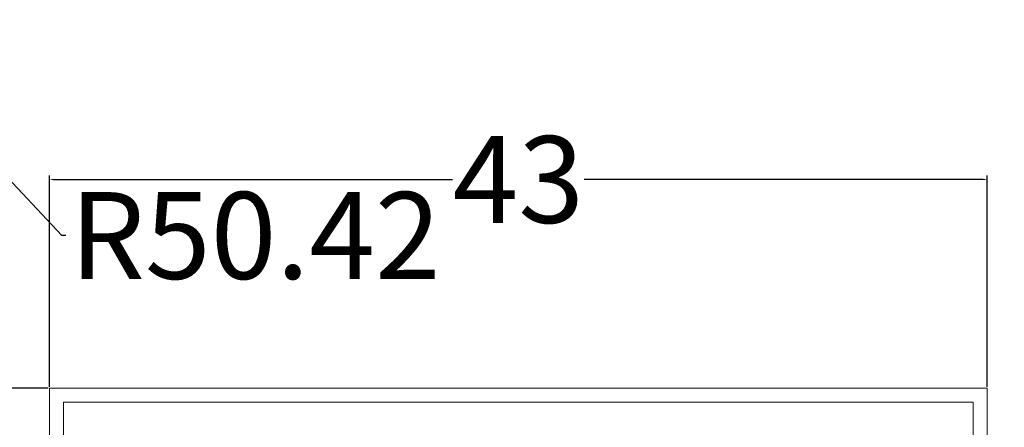
# Model space of a CAD drawing. Units: inches. Extents: x 1291 to 2095, y 532 to 1090.
# Tile 8 of 14: x 1618 to 1663, y 798 to 817. Entities that reach past the tile are written whole.
import ezdxf

# ---------------------------------------------------------------- set-up
doc = ezdxf.new("R2010")
doc.units = ezdxf.units.IN
doc.header["$MEASUREMENT"] = 0
doc.layers.add('A-ANNO-DIMS', color=2, linetype='Continuous', lineweight=18)
doc.layers.add('A-FURN', color=8, linetype='Continuous', lineweight=18)
doc.styles.get("Standard").update_dxf_attribs({"font": 'arial.ttf'})
doc.dimstyles.get("Standard").update_dxf_attribs({"dimtxt": 4, "dimasz": 0.18, "dimexe": 0.18, "dimexo": 0.0625, "dimgap": 0.09, "dimtad": 0, "dimtih": 1, "dimtoh": 1, "dimdec": 0, "dimrnd": 6, "dimzin": 0, "dimdsep": 46, "dimlunit": 3, "dimtxsty": 'Standard', "dimcen": 0.09, "dimadec": 0, "dimazin": 0, "dimtfac": 1, "dimtdec": 0, "dimtofl": 0, "dimtmove": 0, "dimatfit": 3, "dimfxl": 1, "dimtolj": 1, "dimtzin": 0, "dimarcsym": 0})

# ---------------------------------------------------------------- blocks, each defined once
blk = doc.blocks.new('A$C73B76B3A')
for p, q in [((0, 0), (0, 2)), ((1.35, 0), (1.35, 2)), ((0.02, 0.02), (0.02, 1.98)), ((1.33, 1.98), (1.33, 0.02)), ((1.33, 0.02), (0.02, 0.02)), ((1.35, 0), (0, 0))]:
    blk.add_line(p, q)
blk = doc.blocks.new('*D30')
at = {"layer": 'A-ANNO-DIMS', "color": 0, "lineweight": -2, "transparency": 16777216}
for p, q in [((1618.87, 799.814), (1609.145, 799.814)), ((1609.325, 799.634), (1609.325, 769.922)), ((1609.325, 735.946), (1609.325, 765.658)), ((1618.87, 735.766), (1609.145, 735.766))]:
    blk.add_line(p, q, dxfattribs=at)
at = {"layer": 'A-ANNO-DIMS', "color": 0, "transparency": 16777216}
for points in [[(1609.295, 799.634), (1609.355, 799.634), (1609.325, 799.814)], [(1609.295, 735.946), (1609.355, 735.946), (1609.325, 735.766)]]:
    blk.add_solid(points, dxfattribs=at)
at = {"layer": 'Defpoints', "color": 0, "transparency": 16777216}
for p in [(1618.932, 799.814), (1609.325, 735.766), (1618.932, 735.766)]:
    blk.add_point(p, dxfattribs=at)
at = {"layer": 'A-ANNO-DIMS', "color": 0, "transparency": 16777216, "insert": (1609.325, 767.79), "char_height": 4, "attachment_point": 5}
blk.add_mtext('\\A1;BED 64', dxfattribs=at)
blk = doc.blocks.new('*D31')
at = {"layer": 'A-ANNO-DIMS', "color": 0, "lineweight": -2, "transparency": 16777216}
for p, q in [((1618.932, 799.877), (1618.932, 809.602)), ((1619.112, 809.422), (1637.513, 809.422)), ((1661.985, 809.422), (1643.584, 809.422)), ((1662.165, 799.877), (1662.165, 809.602))]:
    blk.add_line(p, q, dxfattribs=at)
at = {"layer": 'A-ANNO-DIMS', "color": 0, "transparency": 16777216}
for points in [[(1619.112, 809.452), (1619.112, 809.392), (1618.932, 809.422)], [(1661.985, 809.452), (1661.985, 809.392), (1662.165, 809.422)]]:
    blk.add_solid(points, dxfattribs=at)
at = {"layer": 'Defpoints', "color": 0, "transparency": 16777216}
for p in [(1618.932, 809.422), (1618.932, 799.814), (1662.165, 799.814)]:
    blk.add_point(p, dxfattribs=at)
at = {"layer": 'A-ANNO-DIMS', "color": 0, "transparency": 16777216, "insert": (1640.548, 809.422), "char_height": 4, "attachment_point": 5}
blk.add_mtext('\\A1;43', dxfattribs=at)
blk = doc.blocks.new('*D46')
at = {"layer": 'A-ANNO-DIMS', "color": 0, "lineweight": -2, "transparency": 16777216}
for p, q in [((1600.27, 579.843), (1600.27, 1087.16)), ((1600.45, 1086.98), (1636.471, 1086.98)), ((1685.404, 1086.98), (1649.383, 1086.98)), ((1685.584, 579.843), (1685.584, 1087.16))]:
    blk.add_line(p, q, dxfattribs=at)
at = {"layer": 'A-ANNO-DIMS', "color": 0, "transparency": 16777216}
for points in [[(1600.45, 1087.01), (1600.45, 1086.95), (1600.27, 1086.98)], [(1685.404, 1087.01), (1685.404, 1086.95), (1685.584, 1086.98)]]:
    blk.add_solid(points, dxfattribs=at)
at = {"layer": 'Defpoints', "color": 0, "transparency": 16777216}
for p in [(1685.584, 1086.98), (1600.27, 579.78), (1685.584, 579.78)]:
    blk.add_point(p, dxfattribs=at)
at = {"layer": 'A-ANNO-DIMS', "color": 0, "transparency": 16777216, "insert": (1642.927, 1086.98), "char_height": 4, "attachment_point": 5}
blk.add_mtext('\\A1;85.31', dxfattribs=at)
blk = doc.blocks.new('*D49')
at = {"layer": 'A-ANNO-DIMS', "color": 0, "lineweight": -2, "transparency": 16777216}
for p, q in [((1694.074, 852.718), (1694.074, 534.4)), ((1586.074, 816.718), (1586.074, 534.4)), ((1586.254, 534.58), (1635.749, 534.58)), ((1693.894, 534.58), (1644.398, 534.58))]:
    blk.add_line(p, q, dxfattribs=at)
at = {"layer": 'A-ANNO-DIMS', "color": 0, "transparency": 16777216}
for points in [[(1586.254, 534.61), (1586.254, 534.55), (1586.074, 534.58)], [(1693.894, 534.61), (1693.894, 534.55), (1694.074, 534.58)]]:
    blk.add_solid(points, dxfattribs=at)
at = {"layer": 'Defpoints', "color": 0, "transparency": 16777216}
for p in [(1694.074, 852.78), (1586.074, 816.78), (1694.074, 534.58)]:
    blk.add_point(p, dxfattribs=at)
at = {"layer": 'A-ANNO-DIMS', "color": 0, "transparency": 16777216, "insert": (1640.074, 534.58), "char_height": 4, "attachment_point": 5}
blk.add_mtext('\\A1;108', dxfattribs=at)
blk = doc.blocks.new('*D51')
at = {"layer": 'A-ANNO-DIMS', "color": 0, "lineweight": -2, "transparency": 16777216}
for p, q in [((1820.011, 852.78), (1297.694, 852.78)), ((1297.874, 852.6), (1297.874, 794.913)), ((1297.874, 732.96), (1297.874, 790.648)), ((1811.011, 732.78), (1297.694, 732.78))]:
    blk.add_line(p, q, dxfattribs=at)
at = {"layer": 'A-ANNO-DIMS', "color": 0, "transparency": 16777216}
for points in [[(1297.844, 852.6), (1297.904, 852.6), (1297.874, 852.78)], [(1297.844, 732.96), (1297.904, 732.96), (1297.874, 732.78)]]:
    blk.add_solid(points, dxfattribs=at)
at = {"layer": 'Defpoints', "color": 0, "transparency": 16777216}
for p in [(1297.874, 852.78), (1820.074, 852.78), (1811.074, 732.78)]:
    blk.add_point(p, dxfattribs=at)
at = {"layer": 'A-ANNO-DIMS', "color": 0, "transparency": 16777216, "insert": (1297.874, 792.78), "char_height": 4, "attachment_point": 5}
blk.add_mtext('\\A1;120', dxfattribs=at)
blk = doc.blocks.new('*D85')
at = {"layer": 'A-ANNO-DIMS', "color": 0, "lineweight": -2, "transparency": 16777216}
for p, q in [((1564.052, 865.509), (1564.232, 865.509)), ((1564.142, 865.419), (1564.142, 865.599)), ((1619.506, 806.844), (1598.868, 828.713)), ((1619.686, 806.844), (1619.506, 806.844))]:
    blk.add_line(p, q, dxfattribs=at)
at = {"layer": 'A-ANNO-DIMS', "color": 0, "transparency": 16777216}
blk.add_solid([(1598.89, 828.733), (1598.846, 828.692), (1598.744, 828.844)], dxfattribs=at)
at = {"layer": 'Defpoints', "color": 0, "transparency": 16777216}
for p in [(1564.142, 865.509), (1598.744, 828.844)]:
    blk.add_point(p, dxfattribs=at)
at = {"layer": 'A-ANNO-DIMS', "color": 0, "transparency": 16777216, "insert": (1628.419, 806.844), "char_height": 4, "attachment_point": 5}
blk.add_mtext('\\A1;R50.42', dxfattribs=at)

msp = doc.modelspace()

# ---------------------------------------------------------------- block references
at = {"layer": 'A-FURN', "xscale": 32.02427574694497, "yscale": 32.02427574694497, "zscale": 32.02427574694497, "rotation": 180}
msp.add_blockref('A$C73B76B3A', (1662.1648, 799.8143), dxfattribs=at)

# ---------------------------------------------------------------- dimensions: what is measured, and where the dimension line sits
at = {"layer": 'A-ANNO-DIMS'}
for base, p1, p2, override, picture, middle in [((1685.5842, 1086.9804), (1600.2697, 579.7804), (1685.5842, 579.7804), {"dimdec": 2, "dimlfac": 1, "dimrnd": 0, "dimzin": 0, "dimdsep": 46, "dimlunit": 2}, '*D46', (1642.927, 1086.9804)), ((1694.0735, 534.5804), (1586.0735, 816.7804), (1694.0735, 852.7804), {"dimdec": 0, "dimlfac": 1, "dimrnd": 0, "dimzin": 0, "dimdsep": 46, "dimlunit": 2}, '*D49', (1640.0735, 534.5804))]:
    dim = msp.add_linear_dim(base=base, p1=p1, p2=p2, dimstyle='Standard', override=override, dxfattribs=at)
    dim.commit()
    dim.dimension.update_dxf_attribs({"geometry": picture, "text_midpoint": middle})
dim = msp.add_radius_dim(center=(1564.1416, 865.5092), mpoint=(1598.7445, 828.8435), dimstyle='Standard', override={"dimdec": 2, "dimlfac": 1, "dimrnd": 0, "dimzin": 0, "dimdsep": 46, "dimlunit": 2}, dxfattribs=at)
dim.commit()
dim.dimension.update_dxf_attribs({"geometry": '*D85', "text_midpoint": (1628.4187, 806.8441), "dimtype": 164})
for base, p1, p2, angle, picture, middle in [((1297.8735, 852.7804), (1811.0735, 732.7804), (1820.0735, 852.7804), 90, '*D51', (1297.8735, 792.7804)), ((1618.932, 809.4216), (1662.1648, 799.8143), (1618.932, 799.8143), 180, '*D31', (1640.5484, 809.4216))]:
    dim = msp.add_linear_dim(base=base, p1=p1, p2=p2, angle=angle, dimstyle='Standard', override={"dimdec": 0, "dimlfac": 1, "dimrnd": 0, "dimzin": 0, "dimdsep": 46, "dimlunit": 2}, dxfattribs=at)
    dim.commit()
    dim.dimension.update_dxf_attribs({"geometry": picture, "text_midpoint": middle})
dim = msp.add_linear_dim(base=(1609.3247, 735.7658), p1=(1618.932, 799.8143), p2=(1618.932, 735.7658), angle=270, text='BED <>', dimstyle='Standard', override={"dimdec": 0, "dimlfac": 1, "dimrnd": 0, "dimzin": 0, "dimdsep": 46, "dimlunit": 2}, dxfattribs=at)
dim.commit()
dim.dimension.update_dxf_attribs({"geometry": '*D30', "text_midpoint": (1609.3247, 767.79)})

doc.saveas('drawing.dxf')
